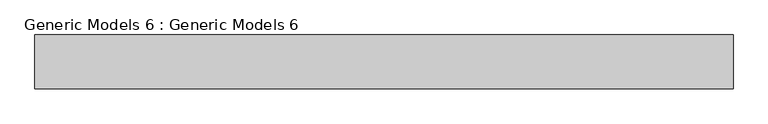
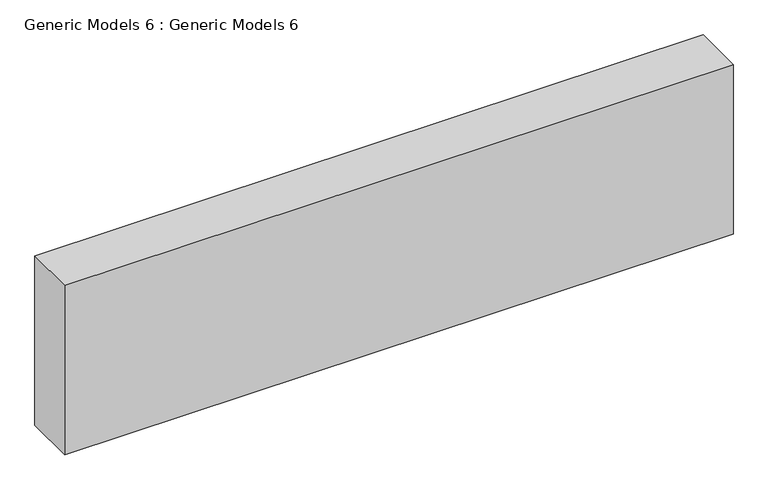
"""IFC4 building model written with IfcOpenShell, lengths in millimetres: proxy geometry, Generic Models 6 : Generic Models 6."""

from ifc_helpers import new_model, si_unit, frame, origin, place, context, project, spatial, polyline, outline, extrude, source, transform, mapped, element, save


def generic_models_6_generic_models_6_a941f71c(model_context):
    return source(origin(), model_context, "Body", "SweptSolid", [
        extrude(outline(polyline([(-5875.9767684, -15333.7742702), (-5875.9767684, -15638.5742702), (-9817.6652876, -15638.5742702), (-9817.6652876, -15333.7742702), (-5875.9767684, -15333.7742702)])), frame((0.0, 0.0, 6400.8), z_axis=(0.0, 0.0, 1.0), x_axis=(1.0, 0.0, 0.0)), (0.0, 0.0, 1.0), 1057.6190549),
    ])


if __name__ == "__main__":
    model = new_model("IFC4")
    model_context = context("Model", 3, world=origin())
    ifc_project = project(units=[si_unit("LENGTHUNIT", "METRE", prefix="MILLI")], contexts=[model_context])
    site = spatial("IfcSite", under=ifc_project)
    building = spatial("IfcBuilding", under=site)
    placement = place(None, origin())
    generic_models_6_generic_models_6_shape = generic_models_6_generic_models_6_a941f71c(model_context)
    element("IfcBuildingElementProxy", 1, Name="Generic Models 6 : Generic Models 6", ObjectType="Generic Models 6 : Generic Models 6", at=placement, inside=building, context=model_context, shape_type="MappedRepresentation", body=[
        mapped(generic_models_6_generic_models_6_shape, transform((0.0, 0.0, 0.0), x_axis=(1.0, 0.0, 0.0), y_axis=(0.0, 1.0, 0.0), z_axis=(0.0, 0.0, 1.0))),
    ])
    save(model, "model.ifc")
